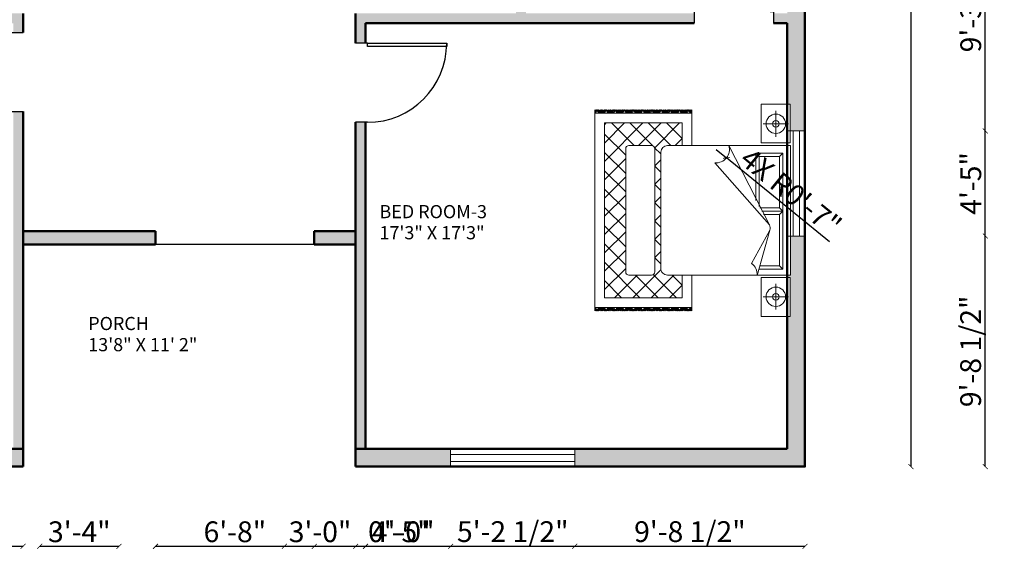
# Model space of a CAD drawing. Units: inches. Extents: x 1549 to 2410, y 1378 to 2139.
# Tile 3 of 6: x 1913 to 2410, y 1378 to 1654. Entities that reach past the tile are written whole.
import ezdxf

# ---------------------------------------------------------------- set-up
doc = ezdxf.new("R2010")
doc.units = ezdxf.units.IN
for name, color, linetype, lineweight in [('A-ANNO-DIMS', 2, 'Continuous', 18), ('A-AREA-IDEN', 7, 'Continuous', 18), ('A-DOOR', 4, 'Continuous', 25), ('A-FURN', 8, 'Continuous', 18), ('A-WALL', 7, 'Continuous', 50), ('WINDOW', 2, 'Continuous', 18)]:
    doc.layers.add(name, color=color, linetype=linetype, lineweight=lineweight)
doc.layers.add('A-WALL-PATT', color=18, linetype='Continuous', lineweight=13, true_color=0x000000)
doc.styles.get("Standard").update_dxf_attribs({"font": 'arial.ttf'})
doc.dimstyles.new('ISO-25', dxfattribs={"dimtxt": 10.5, "dimasz": 2.5, "dimexe": 1.25, "dimexo": 0.625, "dimtad": 1, "dimdec": 0, "dimlunit": 4, "dimtxsty": 'Standard', "dimblk": 'ARCHTICK', "dimcen": 2.5, "dimse1": 1, "dimse2": 1, "dimclrd": 1, "dimclrt": 3, "dimadec": 0, "dimazin": 0, "dimtfac": 1, "dimtdec": 0, "dimtmove": 0, "dimatfit": 3, "dimfxl": 1, "dimarcsym": 0})

# ---------------------------------------------------------------- blocks, each defined once
blk = doc.blocks.new('*U3')
for p, q in [((0, 0), (0, -6)), ((40, 0), (40, -6))]:
    blk.add_line(p, q)
blk.add_lwpolyline([(0, 0), (0, 40), (1.75, 40), (1.75, 0)], close=True)
blk.add_arc((0, 0), 40, 0, 90)
blk = doc.blocks.new('A$C4CB008C5')
for p, q in [((0, 3.019), (0.6, 3.019)), ((0, 2.569), (0, 3.019)), ((0.304, 2.6), (0.304, 2.992)), ((0.6, 3.019), (0.6, 2.569)), ((0.64, 1.121), (0.64, 3.021)), ((0.64, 3.021), (2.64, 3.021)), ((0.64, 2.971), (2.64, 2.971)), ((0.759, 2.905), (2.547, 2.905)), ((0.759, 2.489), (0.759, 2.905)), ((0.759, 2.905), (0.809, 2.855)), ((1.603, 2.855), (1.653, 2.905)), ((1.653, 2.905), (1.653, 2.579)), ((1.653, 2.905), (1.703, 2.855)), ((2.497, 2.855), (2.547, 2.905)), ((2.547, 2.905), (2.547, 2.54)), ((2.64, 3.021), (2.64, 1.121)), ((3.279, 3.019), (2.679, 3.019)), ((2.679, 3.019), (2.679, 2.569)), ((2.975, 2.6), (2.975, 2.992)), ((3.279, 2.569), (3.279, 3.019)), ((0.106, 2.796), (0.503, 2.796)), ((0.809, 2.855), (1.603, 2.855)), ((0.809, 2.539), (0.809, 2.855)), ((1.603, 2.855), (1.603, 2.551)), ((1.703, 2.855), (1.703, 2.607)), ((1.703, 2.855), (2.497, 2.855)), ((2.497, 2.855), (2.497, 2.556)), ((3.174, 2.796), (2.776, 2.796)), ((0.64, 2.071), (1.866, 2.698)), ((0.906, 1.854), (1.866, 2.698)), ((1.946, 2.705), (2.646, 2.507)), ((1.946, 2.705), (2.46, 2.418)), ((0.6, 2.569), (0, 2.569)), ((0.809, 2.539), (0.759, 2.489)), ((1.49, 2.489), (0.759, 2.489)), ((1.58, 2.539), (0.809, 2.539)), ((2.679, 2.569), (3.279, 2.569)), ((0.907, 1.867), (0.919, 1.867)), ((0.09, 1.5), (0.64, 1.5)), ((0.09, 1.491), (0.099, 1.5)), ((0.09, 1.473), (0.116, 1.5)), ((0.09, 1.456), (0.134, 1.5)), ((0.09, 1.474), (0.09, 1.475)), ((0.09, 1.438), (0.126, 1.474)), ((0.117, 1.43), (0.09, 1.457)), ((0.14, 1.389), (0.09, 1.439)), ((0.09, 1.42), (0.099, 1.43)), ((0.14, 1.372), (0.09, 1.422)), ((0.09, 1.368), (0.14, 1.417)), ((0.14, 1.354), (0.09, 1.404)), ((0.09, 1.35), (0.14, 1.4)), ((0.14, 1.336), (0.09, 1.386)), ((0.09, 1.332), (0.14, 1.382)), ((0.14, 1.46), (0.108, 1.492)), ((0.117, 1.412), (0.14, 1.435)), ((0.14, 1.478), (0.118, 1.5)), ((0.14, 1.496), (0.135, 1.5)), ((0.14, 1.442), (0.135, 1.448)), ((0.14, 0), (0.14, 1.5)), ((2.64, 1.5), (3.19, 1.5)), ((3.14, 1.496), (3.144, 1.5)), ((3.14, 1.478), (3.162, 1.5)), ((3.14, 1.5), (3.14, 0)), ((3.14, 1.46), (3.171, 1.492)), ((3.14, 1.442), (3.145, 1.448)), ((3.14, 1.389), (3.19, 1.439)), ((3.162, 1.412), (3.14, 1.435)), ((3.14, 1.372), (3.19, 1.422)), ((3.189, 1.368), (3.14, 1.417)), ((3.14, 1.354), (3.19, 1.404)), ((3.19, 1.35), (3.14, 1.4)), ((3.14, 1.336), (3.19, 1.386)), ((3.19, 1.332), (3.14, 1.382)), ((3.19, 1.456), (3.145, 1.5)), ((3.19, 1.438), (3.154, 1.474)), ((3.162, 1.43), (3.19, 1.457)), ((3.19, 1.473), (3.163, 1.5)), ((3.19, 1.42), (3.18, 1.43)), ((3.19, 1.491), (3.181, 1.5)), ((3.189, 1.474), (3.19, 1.475)), ((0.09, 1.314), (0.14, 1.364)), ((0.09, 1.297), (0.126, 1.333)), ((0.09, 1.333), (0.09, 1.333)), ((0.117, 1.288), (0.09, 1.316)), ((0.14, 1.248), (0.09, 1.298)), ((0.09, 1.279), (0.099, 1.288)), ((0.14, 1.23), (0.09, 1.28)), ((0.09, 1.227), (0.14, 1.276)), ((0.14, 1.213), (0.09, 1.263)), ((0.09, 1.208), (0.14, 1.258)), ((0.14, 1.195), (0.09, 1.245)), ((0.09, 1.19), (0.14, 1.24)), ((0.09, 1.173), (0.14, 1.223)), ((0.14, 1.319), (0.108, 1.35)), ((0.117, 1.271), (0.14, 1.294)), ((0.14, 1.301), (0.135, 1.306)), ((0.29, 1.108), (0.532, 1.35)), ((0.29, 0.15), (0.29, 1.35)), ((0.29, 1.35), (0.64, 1.35)), ((0.674, 0.926), (0.29, 1.31)), ((0.64, 1.243), (0.533, 1.35)), ((2.632, 0.904), (2.99, 1.262)), ((2.64, 1.195), (2.795, 1.35)), ((2.64, 1.35), (2.99, 1.35)), ((2.99, 0.873), (2.64, 1.223)), ((2.99, 1.156), (2.795, 1.35)), ((2.99, 1.35), (2.99, 0.15)), ((3.19, 1.314), (3.14, 1.364)), ((3.14, 1.319), (3.171, 1.35)), ((3.14, 1.301), (3.145, 1.306)), ((3.14, 1.248), (3.19, 1.298)), ((3.162, 1.271), (3.14, 1.294)), ((3.14, 1.23), (3.19, 1.28)), ((3.189, 1.227), (3.14, 1.276)), ((3.14, 1.213), (3.19, 1.263)), ((3.19, 1.208), (3.14, 1.258)), ((3.14, 1.195), (3.19, 1.245)), ((3.19, 1.19), (3.14, 1.24)), ((3.19, 1.173), (3.14, 1.223)), ((3.19, 1.297), (3.154, 1.333)), ((3.162, 1.288), (3.19, 1.316)), ((3.19, 1.279), (3.18, 1.288)), ((3.189, 1.333), (3.19, 1.333)), ((0.09, 1.191), (0.09, 1.192)), ((0.09, 1.155), (0.126, 1.191)), ((0.117, 1.147), (0.09, 1.174)), ((0.14, 1.107), (0.09, 1.157)), ((0.09, 1.137), (0.099, 1.147)), ((0.14, 1.089), (0.09, 1.139)), ((0.09, 1.085), (0.14, 1.134)), ((0.14, 1.071), (0.09, 1.121)), ((0.09, 1.067), (0.14, 1.117)), ((0.14, 1.054), (0.09, 1.104)), ((0.09, 1.049), (0.14, 1.099)), ((0.09, 1.031), (0.14, 1.081)), ((0.14, 1.177), (0.108, 1.209)), ((0.14, 1.036), (0.108, 1.067)), ((0.117, 1.129), (0.14, 1.152)), ((0.14, 1.16), (0.135, 1.165)), ((0.29, 0.825), (0.64, 1.175)), ((3.14, 1.177), (3.171, 1.209)), ((3.14, 1.16), (3.145, 1.165)), ((3.14, 1.107), (3.19, 1.157)), ((3.162, 1.129), (3.14, 1.152)), ((3.14, 1.089), (3.19, 1.139)), ((3.189, 1.085), (3.14, 1.134)), ((3.14, 1.071), (3.19, 1.121)), ((3.19, 1.067), (3.14, 1.117)), ((3.14, 1.054), (3.19, 1.104)), ((3.19, 1.049), (3.14, 1.099)), ((3.19, 1.031), (3.14, 1.081)), ((3.14, 1.036), (3.171, 1.067)), ((3.19, 1.155), (3.154, 1.191)), ((3.162, 1.147), (3.19, 1.174)), ((3.19, 1.137), (3.18, 1.147)), ((3.189, 1.191), (3.19, 1.192)), ((0.09, 1.05), (0.09, 1.051)), ((0.09, 1.014), (0.126, 1.05)), ((0.117, 1.006), (0.09, 1.033)), ((0.14, 0.965), (0.09, 1.015)), ((0.09, 0.996), (0.099, 1.006)), ((0.14, 0.948), (0.09, 0.998)), ((0.09, 0.944), (0.14, 0.993)), ((0.14, 0.93), (0.09, 0.98)), ((0.09, 0.925), (0.14, 0.975)), ((0.14, 0.912), (0.09, 0.962)), ((0.09, 0.908), (0.14, 0.958)), ((0.09, 0.89), (0.14, 0.94)), ((0.14, 0.894), (0.108, 0.926)), ((0.117, 0.988), (0.14, 1.011)), ((0.14, 1.018), (0.135, 1.023)), ((0.64, 0.677), (0.29, 1.027)), ((0.673, 0.925), (0.769, 1.021)), ((0.69, 0.928), (2.59, 0.928)), ((2.54, 1.021), (0.74, 1.021)), ((0.955, 0.928), (0.861, 1.021)), ((0.959, 0.928), (1.052, 1.021)), ((1.238, 0.928), (1.144, 1.021)), ((1.241, 0.928), (1.335, 1.021)), ((1.52, 0.928), (1.427, 1.021)), ((1.524, 0.928), (1.618, 1.021)), ((1.803, 0.928), (1.71, 1.021)), ((1.807, 0.928), (1.9, 1.021)), ((2.086, 0.928), (1.993, 1.021)), ((2.09, 0.928), (2.183, 1.021)), ((2.369, 0.928), (2.276, 1.021)), ((2.373, 0.928), (2.466, 1.021)), ((2.99, 0.59), (2.557, 1.023)), ((2.64, 0.629), (2.99, 0.979)), ((3.14, 1.018), (3.145, 1.023)), ((3.14, 0.965), (3.19, 1.015)), ((3.162, 0.988), (3.14, 1.011)), ((3.14, 0.948), (3.19, 0.998)), ((3.189, 0.944), (3.14, 0.993)), ((3.14, 0.93), (3.19, 0.98)), ((3.19, 0.925), (3.14, 0.975)), ((3.14, 0.912), (3.19, 0.962)), ((3.19, 0.908), (3.14, 0.958)), ((3.19, 0.89), (3.14, 0.94)), ((3.14, 0.894), (3.171, 0.926)), ((3.19, 1.014), (3.154, 1.05)), ((3.162, 1.006), (3.19, 1.033)), ((3.19, 0.996), (3.18, 1.006)), ((3.189, 1.05), (3.19, 1.051)), ((0.09, 0.908), (0.09, 0.909)), ((0.09, 0.872), (0.126, 0.908)), ((0.117, 0.864), (0.09, 0.891)), ((0.14, 0.824), (0.09, 0.874)), ((0.09, 0.855), (0.099, 0.864)), ((0.14, 0.806), (0.09, 0.856)), ((0.09, 0.802), (0.14, 0.852)), ((0.14, 0.788), (0.09, 0.838)), ((0.09, 0.784), (0.14, 0.834)), ((0.14, 0.771), (0.09, 0.821)), ((0.09, 0.766), (0.14, 0.816)), ((0.09, 0.749), (0.14, 0.799)), ((0.09, 0.767), (0.09, 0.768)), ((0.09, 0.731), (0.126, 0.767)), ((0.14, 0.753), (0.108, 0.785)), ((0.117, 0.847), (0.14, 0.869)), ((0.14, 0.877), (0.135, 0.882)), ((0.29, 0.542), (0.643, 0.895)), ((0.64, 0.878), (0.64, 0.528)), ((2.64, 0.878), (2.64, 0.528)), ((3.14, 0.877), (3.145, 0.882)), ((3.14, 0.824), (3.19, 0.874)), ((3.162, 0.847), (3.14, 0.869)), ((3.14, 0.806), (3.19, 0.856)), ((3.189, 0.802), (3.14, 0.852)), ((3.14, 0.788), (3.19, 0.838)), ((3.19, 0.784), (3.14, 0.834)), ((3.14, 0.771), (3.19, 0.821)), ((3.19, 0.766), (3.14, 0.816)), ((3.19, 0.749), (3.14, 0.799)), ((3.14, 0.753), (3.171, 0.785)), ((3.19, 0.872), (3.154, 0.908)), ((3.19, 0.731), (3.154, 0.767)), ((3.162, 0.864), (3.19, 0.891)), ((3.19, 0.855), (3.18, 0.864)), ((3.189, 0.908), (3.19, 0.909)), ((3.189, 0.767), (3.19, 0.768)), ((0.117, 0.723), (0.09, 0.75)), ((0.14, 0.682), (0.09, 0.732)), ((0.09, 0.713), (0.099, 0.723)), ((0.14, 0.665), (0.09, 0.715)), ((0.09, 0.661), (0.14, 0.71)), ((0.14, 0.647), (0.09, 0.697)), ((0.09, 0.642), (0.14, 0.692)), ((0.14, 0.629), (0.09, 0.679)), ((0.09, 0.625), (0.14, 0.675)), ((0.09, 0.607), (0.14, 0.657)), ((0.09, 0.589), (0.126, 0.626)), ((0.09, 0.626), (0.09, 0.626)), ((0.117, 0.581), (0.09, 0.609)), ((0.14, 0.612), (0.108, 0.643)), ((0.117, 0.705), (0.14, 0.728)), ((0.14, 0.735), (0.135, 0.74)), ((0.884, 0.15), (0.29, 0.744)), ((0.29, 0.259), (0.64, 0.609)), ((2.443, 0.15), (2.99, 0.696)), ((2.99, 0.307), (2.64, 0.657)), ((3.14, 0.735), (3.145, 0.74)), ((3.14, 0.682), (3.19, 0.732)), ((3.162, 0.705), (3.14, 0.728)), ((3.14, 0.665), (3.19, 0.715)), ((3.189, 0.661), (3.14, 0.71)), ((3.14, 0.647), (3.19, 0.697)), ((3.19, 0.642), (3.14, 0.692)), ((3.14, 0.629), (3.19, 0.679)), ((3.19, 0.625), (3.14, 0.675)), ((3.19, 0.607), (3.14, 0.657)), ((3.14, 0.612), (3.171, 0.643)), ((3.19, 0.589), (3.154, 0.626)), ((3.162, 0.723), (3.19, 0.75)), ((3.162, 0.581), (3.19, 0.609)), ((3.19, 0.713), (3.18, 0.723)), ((3.189, 0.626), (3.19, 0.626)), ((0.14, 0.541), (0.09, 0.591)), ((0.09, 0.572), (0.099, 0.581)), ((0.14, 0.523), (0.09, 0.573)), ((0.09, 0.519), (0.14, 0.569)), ((0.14, 0.506), (0.09, 0.556)), ((0.09, 0.501), (0.14, 0.551)), ((0.14, 0.488), (0.09, 0.538)), ((0.09, 0.483), (0.14, 0.533)), ((0.09, 0.466), (0.14, 0.516)), ((0.09, 0.484), (0.09, 0.485)), ((0.09, 0.448), (0.126, 0.484)), ((0.117, 0.44), (0.09, 0.467)), ((0.14, 0.47), (0.108, 0.502)), ((0.117, 0.564), (0.14, 0.586)), ((0.14, 0.594), (0.135, 0.599)), ((0.14, 0.453), (0.135, 0.458)), ((0.601, 0.15), (0.29, 0.462)), ((0.463, 0.15), (0.791, 0.478)), ((0.69, 0.478), (2.59, 0.478)), ((0.746, 0.15), (1.074, 0.478)), ((1.167, 0.15), (0.839, 0.478)), ((1.029, 0.15), (1.357, 0.478)), ((1.45, 0.15), (1.122, 0.478)), ((1.312, 0.15), (1.64, 0.478)), ((1.733, 0.15), (1.405, 0.478)), ((1.595, 0.15), (1.923, 0.478)), ((2.016, 0.15), (1.688, 0.478)), ((1.878, 0.15), (2.206, 0.478)), ((2.298, 0.15), (1.97, 0.478)), ((2.16, 0.15), (2.488, 0.478)), ((2.581, 0.15), (2.253, 0.478)), ((2.864, 0.15), (2.536, 0.478)), ((3.14, 0.594), (3.145, 0.599)), ((3.14, 0.541), (3.19, 0.591)), ((3.162, 0.564), (3.14, 0.586)), ((3.14, 0.523), (3.19, 0.573)), ((3.189, 0.519), (3.14, 0.569)), ((3.14, 0.506), (3.19, 0.556)), ((3.19, 0.501), (3.14, 0.551)), ((3.14, 0.488), (3.19, 0.538)), ((3.19, 0.483), (3.14, 0.533)), ((3.19, 0.466), (3.14, 0.516)), ((3.14, 0.47), (3.171, 0.502)), ((3.14, 0.453), (3.145, 0.458)), ((3.19, 0.448), (3.154, 0.484)), ((3.162, 0.44), (3.19, 0.467)), ((3.19, 0.572), (3.18, 0.581)), ((3.189, 0.484), (3.19, 0.485)), ((0.14, 0.399), (0.09, 0.449)), ((0.09, 0.43), (0.099, 0.44)), ((0.14, 0.382), (0.09, 0.432)), ((0.09, 0.378), (0.14, 0.427)), ((0.14, 0.364), (0.09, 0.414)), ((0.09, 0.36), (0.14, 0.41)), ((0.14, 0.346), (0.09, 0.396)), ((0.09, 0.342), (0.14, 0.392)), ((0.09, 0.324), (0.14, 0.374)), ((0.09, 0.307), (0.126, 0.343)), ((0.09, 0.343), (0.09, 0.343)), ((0.117, 0.299), (0.09, 0.326)), ((0.14, 0.258), (0.09, 0.308)), ((0.14, 0.329), (0.108, 0.36)), ((0.117, 0.422), (0.14, 0.445)), ((0.14, 0.311), (0.135, 0.316)), ((2.726, 0.15), (2.99, 0.414)), ((3.14, 0.399), (3.19, 0.449)), ((3.162, 0.422), (3.14, 0.445)), ((3.14, 0.382), (3.19, 0.432)), ((3.189, 0.378), (3.14, 0.427)), ((3.14, 0.364), (3.19, 0.414)), ((3.19, 0.36), (3.14, 0.41)), ((3.14, 0.346), (3.19, 0.396)), ((3.19, 0.342), (3.14, 0.392)), ((3.19, 0.324), (3.14, 0.374)), ((3.14, 0.329), (3.171, 0.36)), ((3.14, 0.311), (3.145, 0.316)), ((3.14, 0.258), (3.19, 0.308)), ((3.19, 0.307), (3.154, 0.343)), ((3.162, 0.299), (3.19, 0.326)), ((3.19, 0.43), (3.18, 0.44)), ((3.189, 0.343), (3.19, 0.343)), ((0.09, 0.289), (0.099, 0.299)), ((0.14, 0.24), (0.09, 0.29)), ((0.09, 0.237), (0.14, 0.286)), ((0.14, 0.223), (0.09, 0.273)), ((0.09, 0.218), (0.14, 0.268)), ((0.14, 0.205), (0.09, 0.255)), ((0.09, 0.201), (0.14, 0.251)), ((0.09, 0.183), (0.14, 0.233)), ((0.09, 0.201), (0.09, 0.202)), ((0.09, 0.165), (0.126, 0.201)), ((0.117, 0.157), (0.09, 0.184)), ((0.14, 0.117), (0.09, 0.167)), ((0.09, 0.148), (0.099, 0.157)), ((0.14, 0.187), (0.108, 0.219)), ((0.117, 0.281), (0.14, 0.304)), ((0.117, 0.139), (0.14, 0.162)), ((0.14, 0.17), (0.135, 0.175)), ((0.318, 0.15), (0.29, 0.179)), ((3.162, 0.281), (3.14, 0.304)), ((3.14, 0.24), (3.19, 0.29)), ((3.189, 0.237), (3.14, 0.286)), ((3.14, 0.223), (3.19, 0.273)), ((3.19, 0.218), (3.14, 0.268)), ((3.14, 0.205), (3.19, 0.255)), ((3.19, 0.201), (3.14, 0.251)), ((3.19, 0.183), (3.14, 0.233)), ((3.14, 0.187), (3.171, 0.219)), ((3.14, 0.17), (3.145, 0.175)), ((3.14, 0.117), (3.19, 0.167)), ((3.162, 0.139), (3.14, 0.162)), ((3.19, 0.165), (3.154, 0.201)), ((3.162, 0.157), (3.19, 0.184)), ((3.19, 0.289), (3.18, 0.299)), ((3.19, 0.148), (3.18, 0.157)), ((3.189, 0.201), (3.19, 0.202)), ((0.14, 0.099), (0.09, 0.149)), ((0.09, 0.095), (0.14, 0.144)), ((0.14, 0.081), (0.09, 0.131)), ((0.09, 0.077), (0.14, 0.127)), ((0.14, 0.064), (0.09, 0.114)), ((0.09, 0.059), (0.14, 0.109)), ((0.09, 0.041), (0.14, 0.091)), ((0.09, 0.06), (0.09, 0.061)), ((0.09, 0.024), (0.126, 0.06)), ((0.117, 0.016), (0.09, 0.043)), ((0.115, 0), (0.09, 0.025)), ((0.09, 0.006), (0.099, 0.016)), ((0.097, 0), (0.09, 0.008)), ((0.14, 0.046), (0.108, 0.078)), ((0.119, 0), (0.14, 0.021)), ((0.14, 0.028), (0.135, 0.033)), ((0.137, 0), (0.14, 0.003)), ((2.99, 0.15), (0.29, 0.15)), ((3.14, 0.099), (3.19, 0.149)), ((3.189, 0.095), (3.14, 0.144)), ((3.14, 0.081), (3.19, 0.131)), ((3.19, 0.077), (3.14, 0.127)), ((3.14, 0.064), (3.19, 0.114)), ((3.19, 0.059), (3.14, 0.109)), ((3.19, 0.041), (3.14, 0.091)), ((3.14, 0.046), (3.171, 0.078)), ((3.14, 0.028), (3.145, 0.033)), ((3.16, 0), (3.14, 0.021)), ((3.143, 0), (3.14, 0.003)), ((3.19, 0.024), (3.154, 0.06)), ((3.162, 0.016), (3.19, 0.043)), ((3.164, 0), (3.19, 0.025)), ((3.19, 0.006), (3.18, 0.016)), ((3.182, 0), (3.19, 0.008)), ((3.189, 0.06), (3.19, 0.061)), ((0.09, 0), (3.19, 0))]:
    blk.add_line(p, q)
for centre, radius in [((0.304, 2.796), 0.15), ((2.975, 2.796), 0.15), ((0.304, 2.796), 0.05), ((2.975, 2.796), 0.05)]:
    blk.add_circle(centre, radius)
for centre, radius, start, end in [((1.915, 2.61), 0.1, 71.7215, 119.0799), ((2.626, 2.31), 0.198, 84.1725, 146.9889), ((0.7, 1.873), 0.207, 354.6422, 106.9775), ((0.74, 1.121), 0.1, 180, 270), ((2.54, 1.121), 0.1, 270, 0), ((0.69, 0.878), 0.05, 90, 180), ((2.59, 0.878), 0.05, 0, 90), ((0.69, 0.528), 0.05, 180, 270), ((2.59, 0.528), 0.05, 270, 0)]:
    blk.add_arc(centre, radius, start, end)
blk = doc.blocks.new('_ArchTick')
at = {"color": 0, "linetype": 'ByBlock', "const_width": 0.15}
blk.add_lwpolyline([(-0.5, -0.5), (0.5, 0.5)], dxfattribs=at)
blk = doc.blocks.new('*D14')
at = {"layer": 'A-ANNO-DIMS', "color": 0, "lineweight": -2, "transparency": 16777216}
blk.add_line((2363.11, 2069.01), (2363.11, 1428.01), dxfattribs=at)
at = {"layer": 'Defpoints', "color": 0, "transparency": 16777216}
for p in [(2309.62, 2069.01), (2309.62, 1428.01), (2363.11, 1428.01)]:
    blk.add_point(p, dxfattribs=at)
at = {"layer": 'A-ANNO-DIMS', "color": 0, "lineweight": -2, "transparency": 16777216, "xscale": 2.5, "yscale": 2.5, "zscale": 2.5}
for p, rotation in [((2363.11, 2069.01), 90), ((2363.11, 1428.01), 270)]:
    blk.add_blockref('_ArchTick', p, dxfattribs=dict(at, rotation=rotation))
at = {"layer": 'A-ANNO-DIMS', "color": 0, "transparency": 16777216, "insert": (2357.12, 1748.51), "char_height": 10.5, "attachment_point": 5, "rotation": 90}
blk.add_mtext('53\'-5"', dxfattribs=at)
blk = doc.blocks.new('*D29')
at = {"layer": 'A-ANNO-DIMS', "color": 1, "lineweight": -2, "transparency": 16777216}
blk.add_line((1815.42, 1387.76), (1914.62, 1387.76), dxfattribs=at)
at = {"layer": 'Defpoints', "color": 0, "transparency": 16777216}
for p in [(1815.42, 1428.01), (1914.62, 1428.01), (1914.62, 1387.76)]:
    blk.add_point(p, dxfattribs=at)
at = {"layer": 'A-ANNO-DIMS', "color": 1, "lineweight": -2, "transparency": 16777216, "xscale": 2.5, "yscale": 2.5, "zscale": 2.5, "rotation": 180}
blk.add_blockref('_ArchTick', (1815.42, 1387.76), dxfattribs=at)
at = {"layer": 'A-ANNO-DIMS', "color": 1, "lineweight": -2, "transparency": 16777216, "xscale": 2.5, "yscale": 2.5, "zscale": 2.5}
blk.add_blockref('_ArchTick', (1914.62, 1387.76), dxfattribs=at)
at = {"layer": 'A-ANNO-DIMS', "color": 3, "transparency": 16777216, "insert": (1865.02, 1393.75), "char_height": 10.5, "attachment_point": 5}
blk.add_mtext('8\'-3"', dxfattribs=at)
blk = doc.blocks.new('*D30')
at = {"layer": 'A-ANNO-DIMS', "color": 1, "lineweight": -2, "transparency": 16777216}
blk.add_line((2082.62, 1387.76), (2130.61, 1387.76), dxfattribs=at)
at = {"layer": 'Defpoints', "color": 0, "transparency": 16777216}
for p in [(2082.62, 1428.01), (2130.61, 1428.01), (2130.61, 1387.76)]:
    blk.add_point(p, dxfattribs=at)
at = {"layer": 'A-ANNO-DIMS', "color": 1, "lineweight": -2, "transparency": 16777216, "xscale": 2.5, "yscale": 2.5, "zscale": 2.5, "rotation": 180}
blk.add_blockref('_ArchTick', (2082.62, 1387.76), dxfattribs=at)
at = {"layer": 'A-ANNO-DIMS', "color": 1, "lineweight": -2, "transparency": 16777216, "xscale": 2.5, "yscale": 2.5, "zscale": 2.5}
blk.add_blockref('_ArchTick', (2130.61, 1387.76), dxfattribs=at)
at = {"layer": 'A-ANNO-DIMS', "color": 3, "transparency": 16777216, "insert": (2106.62, 1393.75), "char_height": 10.5, "attachment_point": 5}
blk.add_mtext('4\'-0"', dxfattribs=at)
blk = doc.blocks.new('*D31')
at = {"layer": 'A-ANNO-DIMS', "color": 1, "lineweight": -2, "transparency": 16777216}
blk.add_line((2130.61, 1387.76), (2193.34, 1387.76), dxfattribs=at)
at = {"layer": 'Defpoints', "color": 0, "transparency": 16777216}
for p in [(2130.61, 1428.01), (2193.34, 1428.01), (2193.34, 1387.76)]:
    blk.add_point(p, dxfattribs=at)
at = {"layer": 'A-ANNO-DIMS', "color": 1, "lineweight": -2, "transparency": 16777216, "xscale": 2.5, "yscale": 2.5, "zscale": 2.5, "rotation": 180}
blk.add_blockref('_ArchTick', (2130.61, 1387.76), dxfattribs=at)
at = {"layer": 'A-ANNO-DIMS', "color": 1, "lineweight": -2, "transparency": 16777216, "xscale": 2.5, "yscale": 2.5, "zscale": 2.5}
blk.add_blockref('_ArchTick', (2193.34, 1387.76), dxfattribs=at)
at = {"layer": 'A-ANNO-DIMS', "color": 3, "transparency": 16777216, "insert": (2161.98, 1393.82), "char_height": 10.5, "attachment_point": 5}
blk.add_mtext('5\'-2 1/2"', dxfattribs=at)
blk = doc.blocks.new('*D32')
at = {"layer": 'A-ANNO-DIMS', "color": 1, "lineweight": -2, "transparency": 16777216}
blk.add_line((2193.34, 1387.76), (2309.62, 1387.76), dxfattribs=at)
at = {"layer": 'Defpoints', "color": 0, "transparency": 16777216}
for p in [(2193.34, 1428.01), (2309.62, 1428.01), (2309.62, 1387.76)]:
    blk.add_point(p, dxfattribs=at)
at = {"layer": 'A-ANNO-DIMS', "color": 1, "lineweight": -2, "transparency": 16777216, "xscale": 2.5, "yscale": 2.5, "zscale": 2.5, "rotation": 180}
blk.add_blockref('_ArchTick', (2193.34, 1387.76), dxfattribs=at)
at = {"layer": 'A-ANNO-DIMS', "color": 1, "lineweight": -2, "transparency": 16777216, "xscale": 2.5, "yscale": 2.5, "zscale": 2.5}
blk.add_blockref('_ArchTick', (2309.62, 1387.76), dxfattribs=at)
at = {"layer": 'A-ANNO-DIMS', "color": 3, "transparency": 16777216, "insert": (2251.48, 1393.82), "char_height": 10.5, "attachment_point": 5}
blk.add_mtext('9\'-8 1/2"', dxfattribs=at)
blk = doc.blocks.new('*D39')
at = {"layer": 'A-ANNO-DIMS', "color": 1, "lineweight": -2, "transparency": 16777216}
blk.add_line((2400.7, 1428.01), (2400.7, 1544.51), dxfattribs=at)
at = {"layer": 'Defpoints', "color": 0, "transparency": 16777216}
for p in [(2309.62, 1544.51), (2400.7, 1544.51), (2309.62, 1428.01)]:
    blk.add_point(p, dxfattribs=at)
at = {"layer": 'A-ANNO-DIMS', "color": 1, "lineweight": -2, "transparency": 16777216, "xscale": 2.5, "yscale": 2.5, "zscale": 2.5}
for p, rotation in [((2400.7, 1544.51), 90), ((2400.7, 1428.01), 270)]:
    blk.add_blockref('_ArchTick', p, dxfattribs=dict(at, rotation=rotation))
at = {"layer": 'A-ANNO-DIMS', "color": 3, "transparency": 16777216, "insert": (2394.65, 1486.26), "char_height": 10.5, "attachment_point": 5, "rotation": 90}
blk.add_mtext('9\'-8 1/2"', dxfattribs=at)
blk = doc.blocks.new('*D40')
at = {"layer": 'A-ANNO-DIMS', "color": 1, "lineweight": -2, "transparency": 16777216}
blk.add_line((2400.7, 1544.51), (2400.7, 1597.64), dxfattribs=at)
at = {"layer": 'Defpoints', "color": 0, "transparency": 16777216}
for p in [(2309.62, 1597.64), (2400.7, 1597.64), (2309.62, 1544.51)]:
    blk.add_point(p, dxfattribs=at)
at = {"layer": 'A-ANNO-DIMS', "color": 1, "lineweight": -2, "transparency": 16777216, "xscale": 2.5, "yscale": 2.5, "zscale": 2.5}
for p, rotation in [((2400.7, 1597.64), 90), ((2400.7, 1544.51), 270)]:
    blk.add_blockref('_ArchTick', p, dxfattribs=dict(at, rotation=rotation))
at = {"layer": 'A-ANNO-DIMS', "color": 3, "transparency": 16777216, "insert": (2394.74, 1571.08), "char_height": 10.5, "attachment_point": 5, "rotation": 90}
blk.add_mtext('4\'-5"', dxfattribs=at)
blk = doc.blocks.new('*D41')
at = {"layer": 'A-ANNO-DIMS', "color": 1, "lineweight": -2, "transparency": 16777216}
blk.add_line((2400.7, 1597.64), (2400.7, 1708.66), dxfattribs=at)
at = {"layer": 'Defpoints', "color": 0, "transparency": 16777216}
for p in [(2309.62, 1708.66), (2400.7, 1708.66), (2309.62, 1597.64)]:
    blk.add_point(p, dxfattribs=at)
at = {"layer": 'A-ANNO-DIMS', "color": 1, "lineweight": -2, "transparency": 16777216, "xscale": 2.5, "yscale": 2.5, "zscale": 2.5}
for p, rotation in [((2400.7, 1708.66), 90), ((2400.7, 1597.64), 270)]:
    blk.add_blockref('_ArchTick', p, dxfattribs=dict(at, rotation=rotation))
at = {"layer": 'A-ANNO-DIMS', "color": 3, "transparency": 16777216, "insert": (2394.71, 1653.15), "char_height": 10.5, "attachment_point": 5, "rotation": 90}
blk.add_mtext('9\'-3"', dxfattribs=at)
blk = doc.blocks.new('*D49')
at = {"layer": 'A-ANNO-DIMS', "color": 1, "lineweight": -2, "transparency": 16777216}
blk.add_line((1981.52, 1387.76), (2061.69, 1387.76), dxfattribs=at)
at = {"layer": 'Defpoints', "color": 0, "transparency": 16777216}
for p in [(1981.52, 1540.24), (2061.69, 1540.24), (2061.69, 1387.76)]:
    blk.add_point(p, dxfattribs=at)
at = {"layer": 'A-ANNO-DIMS', "color": 1, "lineweight": -2, "transparency": 16777216, "xscale": 2.5, "yscale": 2.5, "zscale": 2.5, "rotation": 180}
blk.add_blockref('_ArchTick', (1981.52, 1387.76), dxfattribs=at)
at = {"layer": 'A-ANNO-DIMS', "color": 1, "lineweight": -2, "transparency": 16777216, "xscale": 2.5, "yscale": 2.5, "zscale": 2.5}
blk.add_blockref('_ArchTick', (2061.69, 1387.76), dxfattribs=at)
at = {"layer": 'A-ANNO-DIMS', "color": 3, "transparency": 16777216, "insert": (2021.61, 1393.75), "char_height": 10.5, "attachment_point": 5}
blk.add_mtext('6\'-8"', dxfattribs=at)
blk = doc.blocks.new('*D50')
at = {"layer": 'A-ANNO-DIMS', "color": 1, "lineweight": -2, "transparency": 16777216}
blk.add_line((1923.02, 1387.76), (1963.02, 1387.76), dxfattribs=at)
at = {"layer": 'Defpoints', "color": 0, "transparency": 16777216}
for p in [(1923.02, 1844.01), (1963.02, 1844.01), (1963.02, 1387.76)]:
    blk.add_point(p, dxfattribs=at)
at = {"layer": 'A-ANNO-DIMS', "color": 1, "lineweight": -2, "transparency": 16777216, "xscale": 2.5, "yscale": 2.5, "zscale": 2.5, "rotation": 180}
blk.add_blockref('_ArchTick', (1923.02, 1387.76), dxfattribs=at)
at = {"layer": 'A-ANNO-DIMS', "color": 1, "lineweight": -2, "transparency": 16777216, "xscale": 2.5, "yscale": 2.5, "zscale": 2.5}
blk.add_blockref('_ArchTick', (1963.02, 1387.76), dxfattribs=at)
at = {"layer": 'A-ANNO-DIMS', "color": 3, "transparency": 16777216, "insert": (1943.02, 1393.75), "char_height": 10.5, "attachment_point": 5}
blk.add_mtext('3\'-4"', dxfattribs=at)
blk = doc.blocks.new('*D52')
at = {"layer": 'A-ANNO-DIMS', "color": 1, "lineweight": -2, "transparency": 16777216}
blk.add_line((2046.65, 1387.76), (2082.62, 1387.76), dxfattribs=at)
at = {"layer": 'Defpoints', "color": 0, "transparency": 16777216}
for p in [(2046.65, 1849.01), (2082.62, 1849.01), (2082.62, 1387.76)]:
    blk.add_point(p, dxfattribs=at)
at = {"layer": 'A-ANNO-DIMS', "color": 1, "lineweight": -2, "transparency": 16777216, "xscale": 2.5, "yscale": 2.5, "zscale": 2.5, "rotation": 180}
blk.add_blockref('_ArchTick', (2046.65, 1387.76), dxfattribs=at)
at = {"layer": 'A-ANNO-DIMS', "color": 1, "lineweight": -2, "transparency": 16777216, "xscale": 2.5, "yscale": 2.5, "zscale": 2.5}
blk.add_blockref('_ArchTick', (2082.62, 1387.76), dxfattribs=at)
at = {"layer": 'A-ANNO-DIMS', "color": 3, "transparency": 16777216, "insert": (2064.64, 1393.75), "char_height": 10.5, "attachment_point": 5}
blk.add_mtext('3\'-0"', dxfattribs=at)
blk = doc.blocks.new('*D56')
at = {"layer": 'A-ANNO-DIMS', "color": 1, "lineweight": -2, "transparency": 16777216}
for p, q in [((2082.62, 1387.76), (2087.62, 1387.76)), ((2087.62, 1387.76), (2119.28, 1387.76))]:
    blk.add_line(p, q, dxfattribs=at)
at = {"layer": 'Defpoints', "color": 0, "transparency": 16777216}
for p in [(2082.62, 1849.01), (2087.62, 1849.01), (2087.62, 1387.76)]:
    blk.add_point(p, dxfattribs=at)
at = {"layer": 'A-ANNO-DIMS', "color": 1, "lineweight": -2, "transparency": 16777216, "xscale": 2.5, "yscale": 2.5, "zscale": 2.5, "rotation": 180}
blk.add_blockref('_ArchTick', (2082.62, 1387.76), dxfattribs=at)
at = {"layer": 'A-ANNO-DIMS', "color": 1, "lineweight": -2, "transparency": 16777216, "xscale": 2.5, "yscale": 2.5, "zscale": 2.5}
blk.add_blockref('_ArchTick', (2087.62, 1387.76), dxfattribs=at)
at = {"layer": 'A-ANNO-DIMS', "color": 3, "transparency": 16777216, "insert": (2104.7, 1393.75), "char_height": 10.5, "attachment_point": 5}
blk.add_mtext('0\'-5"', dxfattribs=at)
blk = doc.blocks.new('*D68')
at = {"layer": 'A-ANNO-DIMS', "color": 1, "lineweight": -2, "transparency": 16777216}
for p in [(2264.69, 1588.27), (2322.02, 1541.53)]:
    blk.add_line(p, (2269.94, 1583.99), dxfattribs=at)
at = {"layer": 'Defpoints', "color": 0, "transparency": 16777216}
for p in [(2264.69, 1588.27), (2269.94, 1583.99)]:
    blk.add_point(p, dxfattribs=at)
at = {"layer": 'A-ANNO-DIMS', "color": 1, "lineweight": -2, "transparency": 16777216, "xscale": 2.5, "yscale": 2.5, "zscale": 2.5, "rotation": 140.8118096562743}
blk.add_blockref('_ArchTick', (2269.94, 1583.99), dxfattribs=at)
at = {"layer": 'A-ANNO-DIMS', "color": 3, "transparency": 16777216, "insert": (2301.7, 1565.82), "char_height": 10.5, "attachment_point": 5, "rotation": 320.8118}
blk.add_mtext('4X R0\'-7"', dxfattribs=at)

msp = doc.modelspace()

# ---------------------------------------------------------------- hatches: boundary and pattern name
at = {"layer": 'A-WALL-PATT'}
h = msp.add_hatch(color=256, dxfattribs=at)
h.dxf.hatch_style = 1
h.paths.add_polyline_path([(1760, 2069.01), (1688.62, 2069.01), (1688.62, 2003.68), (1697.62, 2003.68), (1697.62, 2060.01), (1760, 2060.01)])
h.paths.add_polyline_path([(2309.62, 2069.01), (1807.68, 2069.01), (1807.68, 2060.01), (1909.62, 2060.01), (1909.62, 2040.27), (1914.62, 2040.27), (1914.62, 2060.01), (2082.62, 2060.01), (2082.62, 2043.41), (2087.62, 2043.41), (2087.62, 2060.01), (2300.62, 2060.01), (2300.62, 2006.22), (2309.62, 2006.22)])
h.paths.add_polyline_path([(1914.62, 1607.36), (1909.62, 1607.36), (1909.62, 1437.01), (1914.62, 1437.01)])
h.paths.add_polyline_path([(1697.62, 1536.06), (1688.62, 1536.06), (1688.62, 1428.01), (1745.28, 1428.01), (1745.28, 1437.01), (1697.62, 1437.01)])
h.paths.add_polyline_path([(2130.61, 1437.01), (2082.62, 1437.01), (2082.62, 1428.01), (2130.61, 1428.01)])
h.paths.add_polyline_path([(2309.62, 1544.51), (2302.25, 1544.51), (2302.25, 1524.81), (2300.62, 1524.81), (2300.62, 1523.51), (2302.17, 1523.51), (2302.17, 1503.88), (2300.62, 1503.88), (2300.62, 1437.01), (2193.34, 1437.01), (2193.34, 1428.01), (2309.62, 1428.01)])
h.paths.add_polyline_path([(2309.62, 1708.66), (2300.62, 1708.66), (2300.62, 1657.01), (2293.7, 1657.01), (2293.7, 1652.01), (2300.62, 1652.01), (2300.62, 1611.18), (2302.17, 1611.18), (2302.17, 1597.64), (2309.62, 1597.64)])
h.paths.add_polyline_path([(2309.62, 1777.38), (2300.62, 1777.38), (2300.62, 1737.9), (2309.62, 1737.9)])
h.paths.add_polyline_path([(2300.62, 1757.01), (2168.62, 1757.01), (2168.62, 1795.96), (2163.62, 1795.96), (2163.62, 1657.01), (2082.62, 1657.01), (2082.62, 1641.99), (2087.62, 1641.99), (2087.62, 1652.01), (2253.7, 1652.01), (2253.7, 1657.01), (2168.62, 1657.01), (2168.62, 1752.01), (2300.62, 1752.01)])
h.paths.add_polyline_path([(2309.62, 1957.79), (2300.62, 1957.79), (2300.62, 1935.33), (2300.62, 1824.93), (2309.62, 1824.93)])
h.paths.add_polyline_path([(2300.62, 1849.01), (2137.17, 1849.01), (2137.17, 1844.01), (2163.62, 1844.01), (2163.62, 1835.96), (2168.62, 1835.96), (2168.62, 1844.01), (2300.62, 1844.01)])
h.paths.add_polyline_path([(2211.06, 1800.23), (2261.76, 1800.23), (2261.76, 1810.41), (2211.06, 1810.41)], flags=9)
h.paths.add_polyline_path([(2211.1, 1811.05), (2239.18, 1811.05), (2239.18, 1821.02), (2211.1, 1821.02)], flags=9)
h.paths.add_polyline_path([(2187.84, 1718.73), (2233.38, 1718.73), (2233.38, 1728.91), (2187.84, 1728.91)], flags=25)
h.paths.add_polyline_path([(2187.88, 1729.56), (2215.96, 1729.56), (2215.96, 1739.52), (2187.88, 1739.52)], flags=25)
h.paths.add_polyline_path([(1720.01, 1609.74), (1775.87, 1609.74), (1775.87, 1619.93), (1720.01, 1619.93)], flags=9)
h.paths.add_polyline_path([(1719.99, 1620.4), (1782.23, 1620.4), (1782.23, 1630.72), (1719.99, 1630.72)], flags=9)
h.paths.add_polyline_path([(2092.97, 1541.04), (2148.83, 1541.04), (2148.83, 1551.23), (2092.97, 1551.23)], flags=9)
h.paths.add_polyline_path([(2092.94, 1551.69), (2155.19, 1551.69), (2155.19, 1562.02), (2092.94, 1562.02)], flags=9)
h.paths.add_polyline_path([(1759.73, 1747.67), (1815.59, 1747.67), (1815.59, 1757.85), (1759.73, 1757.85)], flags=9)
h.paths.add_polyline_path([(1759.71, 1758.32), (1790.48, 1758.32), (1790.48, 1768.63), (1759.71, 1768.63)], flags=9)
h.paths.add_polyline_path([(1940.79, 1793.43), (1996.65, 1793.43), (1996.65, 1803.61), (1940.79, 1803.61)], flags=9)
h.paths.add_polyline_path([(1940.77, 1804.08), (2006.11, 1804.08), (2006.11, 1814.4), (1940.77, 1814.4)], flags=9)
h.paths.add_polyline_path([(2094.62, 1963.23), (2150.43, 1963.23), (2150.43, 1973.25), (2094.62, 1973.25)], flags=9)
h.paths.add_polyline_path([(2094.57, 1973.75), (2156.81, 1973.75), (2156.81, 1984.07), (2094.57, 1984.07)], flags=9)
h.paths.add_polyline_path([(1943.36, 1930.19), (2000.28, 1930.19), (2000.28, 1940.37), (1943.36, 1940.37)], flags=9)
h.paths.add_polyline_path([(1943.34, 1940.85), (1987.53, 1940.85), (1987.53, 1951.15), (1943.34, 1951.15)], flags=9)
h.paths.add_polyline_path([(1803.94, 1971.5), (1857.22, 1971.5), (1857.22, 1981.68), (1803.94, 1981.68)], flags=9)
h.paths.add_polyline_path([(1803.92, 1982.16), (1866.16, 1982.16), (1866.16, 1992.47), (1803.92, 1992.47)], flags=9)
h = msp.add_hatch(color=256, dxfattribs=at)
h.dxf.hatch_style = 1
h.paths.add_polyline_path([(1697.62, 1844.01), (1688.62, 1844.01), (1688.62, 1657.01), (1697.62, 1657.01)])
h.paths.add_polyline_path([(1697.62, 1955.9), (1688.62, 1955.9), (1688.62, 1844.01), (1697.62, 1844.01), (1867.86, 1844.01), (1867.86, 1849.01), (1697.62, 1849.01)])
h.paths.add_polyline_path([(1697.62, 1652.01), (1909.62, 1652.01), (1909.62, 1647.36), (1914.62, 1647.36), (1914.62, 1657.01), (1697.62, 1657.01), (1688.62, 1657.01), (1688.62, 1584.55), (1697.62, 1584.55)])
h.paths.add_polyline_path([(2087.62, 1601.99), (2082.62, 1601.99), (2082.62, 1437.01), (2087.62, 1437.01)])
h.paths.add_polyline_path([(1981.52, 1547.01), (1914.62, 1547.01), (1914.62, 1540.24), (1981.52, 1540.24)])
h.paths.add_polyline_path([(2082.62, 1547.01), (2061.69, 1547.01), (2061.69, 1540.24), (2082.62, 1540.24)])
h = msp.add_hatch(color=256, dxfattribs=at)
h.dxf.hatch_style = 1
h.paths.add_polyline_path([(1914.62, 1437.01), (1815.42, 1437.01), (1815.42, 1428.01), (1914.62, 1428.01)])

# ---------------------------------------------------------------- linework, layer by layer
at = {"layer": 'A-DOOR'}
msp.add_line((2061.69, 1540.24), (1981.52, 1540.24), dxfattribs=at)
at = {"layer": 'A-WALL'}
for p, q in [((1914.62, 1647.36), (1914.62, 1657.01)), ((2082.62, 1641.99), (2082.62, 1657.01)), ((2087.62, 1652.01), (2253.7, 1652.01)), ((2087.62, 1641.99), (2087.62, 1652.01)), ((2293.7, 1652.01), (2300.62, 1652.01)), ((2300.62, 1652.01), (2300.62, 1437.01)), ((1914.62, 1437.01), (1914.62, 1607.36)), ((2082.62, 1437.01), (2082.62, 1601.99)), ((2087.62, 1437.01), (2087.62, 1601.99)), ((1914.62, 1547.01), (1981.52, 1547.01)), ((1981.52, 1547.01), (1981.52, 1540.24)), ((2061.69, 1547.01), (2082.62, 1547.01)), ((2061.69, 1547.01), (2061.69, 1540.24)), ((1981.52, 1540.24), (1914.62, 1540.24)), ((2061.69, 1540.24), (2082.62, 1540.24)), ((1914.62, 1437.01), (1697.62, 1437.01)), ((1914.62, 1437.01), (1914.62, 1428.01)), ((2300.62, 1437.01), (2082.62, 1437.01)), ((2082.62, 1437.01), (2082.62, 1428.01))]:
    msp.add_line(p, q, dxfattribs=at)
msp.add_lwpolyline([(1914.62, 1428.01), (1688.62, 1428.01), (1688.62, 2069.01), (2309.62, 2069.01), (2309.62, 1428.01), (2082.62, 1428.01)], dxfattribs=at)
at = {"layer": 'WINDOW'}
for p, q in [((2309.62, 1597.64), (2300.62, 1597.64)), ((2300.62, 1597.64), (2300.62, 1544.51)), ((2300.62, 1544.51), (2300.62, 1597.64)), ((2303.61, 1544.51), (2303.61, 1597.64)), ((2306.83, 1544.51), (2306.83, 1597.64)), ((2309.62, 1544.51), (2309.62, 1597.64)), ((2300.62, 1544.51), (2309.62, 1544.51)), ((2130.61, 1437.01), (2130.61, 1428.01)), ((2193.34, 1437.01), (2130.61, 1437.01)), ((2193.34, 1434.1), (2130.61, 1434.1)), ((2193.34, 1428.01), (2193.34, 1437.01)), ((2193.34, 1430.65), (2130.61, 1430.65)), ((2130.61, 1428.01), (2193.34, 1428.01))]:
    msp.add_line(p, q, dxfattribs=at)

# ---------------------------------------------------------------- block references
at = {"layer": 'A-DOOR', "xscale": -1}
msp.add_blockref('*U3', (2293.7, 1658.01), dxfattribs=at)
at = {"layer": 'A-DOOR', "xscale": -1, "rotation": 90}
msp.add_blockref('*U3', (1908.62, 1647.36), dxfattribs=at)
at = {"layer": 'A-DOOR', "rotation": 270}
msp.add_blockref('*U3', (2088.62, 1641.99), dxfattribs=at)
at = {"layer": 'A-FURN', "xscale": 32.72052747801291, "yscale": 32.72052747801291, "zscale": 32.72052747801291, "rotation": 270}
msp.add_blockref('A$C4CB008C5', (2203.4, 1611.18), dxfattribs=at)

# ---------------------------------------------------------------- texts
at = {"layer": 'A-AREA-IDEN'}
for s, height, p in [('BED ROOM-3', 6.645, (2094.66, 1553.53)), ('17\'3" X 17\'3"', 6.6455, (2094.66, 1542.86)), ('PORCH', 6.645, (1947.55, 1497)), ('13\'8" X 11\' 2"', 6.6455, (1947.55, 1486.32))]:
    msp.add_text(s, height=height, dxfattribs=at).set_placement(p)

# ---------------------------------------------------------------- dimensions: what is measured, and where the dimension line sits
at = {"layer": 'A-ANNO-DIMS'}
for base, p1, p2, override, picture, middle in [((2363.11, 1428.01), (2309.62, 2069.01), (2309.62, 1428.01), {"dimclrd": 0, "dimclre": 0, "dimclrt": 0}, '*D14', (2357.12, 1748.51)), ((2400.7, 1708.66), (2309.62, 1597.64), (2309.62, 1708.66), {"dimdec": 1, "dimlfac": 1, "dimrnd": 0, "dimzin": 1, "dimdsep": 46, "dimlunit": 4, "dimfrac": 2}, '*D41', (2394.71, 1653.15)), ((2400.7, 1597.64), (2309.62, 1544.51), (2309.62, 1597.64), {"dimdec": 1, "dimlfac": 1, "dimrnd": 0, "dimzin": 1, "dimdsep": 46, "dimlunit": 4, "dimfrac": 2}, '*D40', (2394.74, 1571.08)), ((2400.7, 1544.51), (2309.62, 1428.01), (2309.62, 1544.51), {"dimdec": 1, "dimlfac": 1, "dimrnd": 0, "dimzin": 1, "dimdsep": 46, "dimlunit": 4, "dimfrac": 2}, '*D39', (2394.65, 1486.26))]:
    dim = msp.add_linear_dim(base=base, p1=p1, p2=p2, angle=90, dimstyle='ISO-25', override=override, dxfattribs=at)
    dim.commit()
    dim.dimension.update_dxf_attribs({"geometry": picture, "text_midpoint": middle})
for base, p1, p2, picture, middle in [((2082.62, 1387.76), (2046.65, 1849.01), (2082.62, 1849.01), '*D52', (2064.64, 1393.75)), ((2087.62, 1387.76), (2082.62, 1849.01), (2087.62, 1849.01), '*D56', (2104.7, 1393.75)), ((1963.02, 1387.76), (1923.02, 1844.01), (1963.02, 1844.01), '*D50', (1943.02, 1393.75)), ((2061.69, 1387.76), (1981.52, 1540.24), (2061.69, 1540.24), '*D49', (2021.61, 1393.75)), ((1914.62, 1387.76), (1815.42, 1428.01), (1914.62, 1428.01), '*D29', (1865.02, 1393.75)), ((2130.61, 1387.76), (2082.62, 1428.01), (2130.61, 1428.01), '*D30', (2106.62, 1393.75)), ((2193.34, 1387.76), (2130.61, 1428.01), (2193.34, 1428.01), '*D31', (2161.98, 1393.82)), ((2309.62, 1387.76), (2193.34, 1428.01), (2309.62, 1428.01), '*D32', (2251.48, 1393.82))]:
    dim = msp.add_linear_dim(base=base, p1=p1, p2=p2, dimstyle='ISO-25', override={"dimdec": 1, "dimlfac": 1, "dimrnd": 0, "dimzin": 1, "dimdsep": 46, "dimlunit": 4, "dimfrac": 2}, dxfattribs=at)
    dim.commit()
    dim.dimension.update_dxf_attribs({"geometry": picture, "text_midpoint": middle})
dim = msp.add_radius_dim(center=(2264.69, 1588.27), mpoint=(2269.94, 1583.99), text='4X <>', dimstyle='ISO-25', override={"dimdec": 1, "dimlfac": 1, "dimrnd": 0, "dimzin": 1, "dimdsep": 46, "dimlunit": 4, "dimfrac": 2}, dxfattribs=at)
dim.commit()
dim.dimension.update_dxf_attribs({"geometry": '*D68', "text_midpoint": (2301.7, 1565.82)})

doc.saveas('drawing.dxf')
